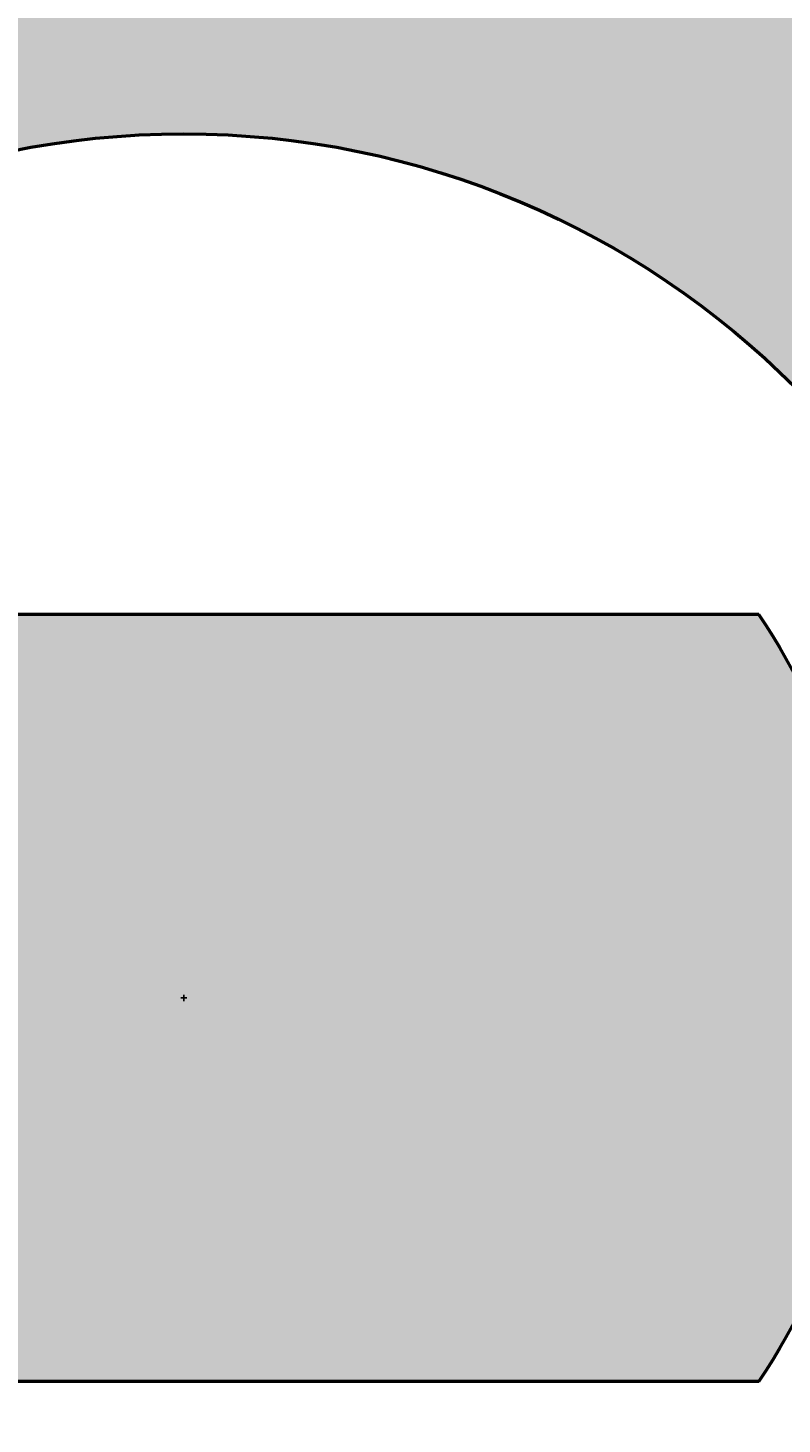
# Model space of a CAD drawing. Units: inches. Extents: x 139261 to 139415, y 52839 to 52963.
# Tile 14 of 20: x 139336 to 139358, y 52888 to 52928. Entities that reach past the tile are written whole.
import ezdxf

# ---------------------------------------------------------------- set-up
doc = ezdxf.new("R2010")
doc.units = ezdxf.units.IN
doc.header["$MEASUREMENT"] = 0
for name, color, linetype, lineweight in [('M-DIMS', 2, 'Continuous', 25), ('M-HATC', 8, 'Continuous', 18), ('M-OUTL', 7, 'Continuous', 50)]:
    doc.layers.add(name, color=color, linetype=linetype, lineweight=lineweight)
doc.styles.get("Standard").update_dxf_attribs({"font": 'arial.ttf'})
doc.dimstyles.get("Standard").update_dxf_attribs({"dimtxt": 0.18, "dimasz": 0.18, "dimexe": 0.18, "dimexo": 0.0625, "dimgap": 0.09, "dimtad": 0, "dimtih": 1, "dimtoh": 1, "dimdec": 4, "dimzin": 0, "dimdsep": 46, "dimtxsty": 'Standard', "dimcen": 0.09, "dimadec": 0, "dimazin": 0, "dimtfac": 1, "dimtdec": 4, "dimtofl": 0, "dimtmove": 0, "dimatfit": 3, "dimfxl": 1, "dimtolj": 1, "dimtzin": 0, "dimarcsym": 0})

# ---------------------------------------------------------------- blocks, each defined once
blk = doc.blocks.new('*D3')
at = {"layer": 'Defpoints', "color": 0, "transparency": 16777216}
for p in [(139359.484, 52906.062), (139321.23, 52894.373)]:
    blk.add_point(p, dxfattribs=at)
at = {"layer": 'M-DIMS', "color": 0, "lineweight": -2, "transparency": 16777216}
for p, q in [((139412.091, 52922.136), (139359.656, 52906.115)), ((139412.271, 52922.136), (139412.091, 52922.136)), ((139340.357, 52900.127), (139340.357, 52900.307)), ((139340.267, 52900.217), (139340.447, 52900.217))]:
    blk.add_line(p, q, dxfattribs=at)
at = {"layer": 'M-DIMS', "color": 0, "transparency": 16777216}
blk.add_solid([(139359.647, 52906.143), (139359.665, 52906.086), (139359.484, 52906.062)], dxfattribs=at)
at = {"layer": 'M-DIMS', "color": 0, "transparency": 16777216, "insert": (139412.902, 52922.136), "char_height": 0.18, "attachment_point": 5}
blk.add_mtext('\\A1;∅40.0000', dxfattribs=at)
blk = doc.blocks.new('*D4')
at = {"layer": 'Defpoints', "color": 0, "transparency": 16777216}
for p in [(139373.053, 52923.26), (139307.661, 52877.175)]:
    blk.add_point(p, dxfattribs=at)
at = {"layer": 'M-DIMS', "color": 0, "lineweight": -2, "transparency": 16777216}
for p, q in [((139414.011, 52952.126), (139373.2, 52923.364)), ((139414.191, 52952.126), (139414.011, 52952.126)), ((139340.357, 52900.127), (139340.357, 52900.307)), ((139340.267, 52900.217), (139340.447, 52900.217))]:
    blk.add_line(p, q, dxfattribs=at)
blk.add_arc((139340.357, 52900.217), 40, 34.9168, 52.0771, dxfattribs=at)
at = {"layer": 'M-DIMS', "color": 0, "transparency": 16777216}
blk.add_solid([(139373.183, 52923.388), (139373.217, 52923.339), (139373.053, 52923.26)], dxfattribs=at)
at = {"layer": 'M-DIMS', "color": 0, "transparency": 16777216, "insert": (139414.822, 52952.126), "char_height": 0.18, "attachment_point": 5}
blk.add_mtext('\\A1;∅80.0000', dxfattribs=at)
blk = doc.blocks.new('*D5')
at = {"layer": 'Defpoints', "color": 0, "transparency": 16777216}
for p in [(139316.763, 52908.484), (139363.951, 52891.951)]:
    blk.add_point(p, dxfattribs=at)
at = {"layer": 'M-DIMS', "color": 0, "lineweight": -2, "transparency": 16777216}
for p, q in [((139262.553, 52927.414), (139262.733, 52927.414)), ((139262.733, 52927.414), (139316.593, 52908.544)), ((139340.357, 52900.127), (139340.357, 52900.307)), ((139340.267, 52900.217), (139340.447, 52900.217))]:
    blk.add_line(p, q, dxfattribs=at)
at = {"layer": 'M-DIMS', "color": 0, "transparency": 16777216}
blk.add_solid([(139316.603, 52908.572), (139316.583, 52908.515), (139316.763, 52908.484)], dxfattribs=at)
at = {"layer": 'M-DIMS', "color": 0, "transparency": 16777216, "insert": (139261.922, 52927.414), "char_height": 0.18, "attachment_point": 5}
blk.add_mtext('\\A1;∅50.0000', dxfattribs=at)
blk = doc.blocks.new('*D6')
at = {"layer": 'Defpoints', "color": 0, "transparency": 16777216}
for p in [(139332.153, 52949.54), (139348.561, 52850.895)]:
    blk.add_point(p, dxfattribs=at)
at = {"layer": 'M-DIMS', "color": 0, "lineweight": -2, "transparency": 16777216}
for p, q in [((139329.787, 52962.682), (139329.967, 52962.682)), ((139329.967, 52962.682), (139332.124, 52949.717)), ((139340.357, 52900.127), (139340.357, 52900.307)), ((139340.267, 52900.217), (139340.447, 52900.217))]:
    blk.add_line(p, q, dxfattribs=at)
at = {"layer": 'M-DIMS', "color": 0, "transparency": 16777216}
blk.add_solid([(139332.153, 52949.722), (139332.094, 52949.713), (139332.153, 52949.54)], dxfattribs=at)
at = {"layer": 'M-DIMS', "color": 0, "transparency": 16777216, "insert": (139329.086, 52962.682), "char_height": 0.18, "attachment_point": 5}
blk.add_mtext('\\A1;∅100.0000', dxfattribs=at)
blk = doc.blocks.new('*D9')
at = {"layer": 'Defpoints', "color": 0, "transparency": 16777216}
for p in [(139302.054, 52932.357), (139378.659, 52868.078)]:
    blk.add_point(p, dxfattribs=at)
at = {"layer": 'M-DIMS', "color": 0, "lineweight": -2, "transparency": 16777216}
for p, q in [((139278.893, 52951.64), (139279.073, 52951.64)), ((139279.073, 52951.64), (139301.916, 52932.472)), ((139340.357, 52900.127), (139340.357, 52900.307)), ((139340.267, 52900.217), (139340.447, 52900.217))]:
    blk.add_line(p, q, dxfattribs=at)
at = {"layer": 'M-DIMS', "color": 0, "transparency": 16777216}
blk.add_solid([(139301.936, 52932.495), (139301.897, 52932.449), (139302.054, 52932.357)], dxfattribs=at)
at = {"layer": 'M-DIMS', "color": 0, "transparency": 16777216, "insert": (139278.506, 52951.64), "char_height": 0.18, "attachment_point": 5}
blk.add_mtext('\\A1;∅100', dxfattribs=at)
blk = doc.blocks.new('*D10')
at = {"layer": 'Defpoints', "color": 0, "transparency": 16777216}
for p in [(139325.07, 52937.181), (139355.644, 52863.254)]:
    blk.add_point(p, dxfattribs=at)
at = {"layer": 'M-DIMS', "color": 0, "lineweight": -2, "transparency": 16777216}
for p, q in [((139340.357, 52900.127), (139340.357, 52900.307)), ((139340.267, 52900.217), (139340.447, 52900.217)), ((139364.816, 52841.075), (139355.712, 52863.087)), ((139364.996, 52841.075), (139364.816, 52841.075))]:
    blk.add_line(p, q, dxfattribs=at)
at = {"layer": 'M-DIMS', "color": 0, "transparency": 16777216}
blk.add_solid([(139355.74, 52863.099), (139355.685, 52863.076), (139355.644, 52863.254)], dxfattribs=at)
at = {"layer": 'M-DIMS', "color": 0, "transparency": 16777216, "insert": (139365.312, 52841.075), "char_height": 0.18, "attachment_point": 5}
blk.add_mtext('\\A1;∅80', dxfattribs=at)

msp = doc.modelspace()

# ---------------------------------------------------------------- hatches: boundary and pattern name
at = {"layer": 'M-HATC'}
h = msp.add_hatch(color=256, dxfattribs=at)
h.dxf.hatch_style = 1
h.paths.add_polyline_path([(139290.35689, 52900.21749, 1), (139390.35689, 52900.21749, 1)])
h.paths.add_polyline_path([(139335.36666, 52939.90499, -0.01563646), (139335.35689, 52940.21749, -1), (139345.35689, 52940.21749, -0.01563646), (139345.34711, 52939.90499, -0.13461315), (139364.89157, 52931.80941, -0.691035), (139373.64116, 52928.50176, -0.21521822), (139371.94881, 52924.75216, -0.13461315), (139380.04439, 52905.20771, -0.43265224), (139385.35689, 52900.21749, -0.43265224), (139380.04439, 52895.22726, -0.13461315), (139371.94881, 52875.68281, -0.21521822), (139373.64116, 52871.93321, -0.691035), (139364.89157, 52868.62556, -0.13461315), (139345.34711, 52860.52999, -0.01563646), (139345.35689, 52860.21749, -1), (139335.35689, 52860.21749, -0.01563646), (139335.36666, 52860.52999, -0.13461315), (139315.82221, 52868.62556, -0.691035), (139307.07262, 52871.93321, -0.21521822), (139308.76496, 52875.68281, -0.13461315), (139300.66939, 52895.22726, -0.43265224), (139295.35689, 52900.21749, -0.43265224), (139300.66939, 52905.20771, -0.13461315), (139308.76496, 52924.75216, -0.21521822), (139307.07262, 52928.50176, -0.691035), (139315.82221, 52931.80941, -0.13461315)], flags=16)
h.paths.add_polyline_path([(139365.35689, 52900.21749, -1), (139315.35689, 52900.21749, -1)], flags=0)
h.paths.add_polyline_path([(139323.71474, 52911.30978), (139356.99903, 52911.30978, -0.3027197), (139356.99903, 52889.12519), (139323.71474, 52889.12519, -0.3027197)], flags=0)
h.paths.add_polyline_path([(139364.89157, 52931.80941, 0.13461315), (139345.34711, 52939.90499, -0.93933644), (139335.36666, 52939.90499, 0.13461315), (139315.82221, 52931.80941, -0.18270763), (139317.07262, 52928.50176, -0.64579494), (139308.76496, 52924.75216, 0.13461315), (139300.66939, 52905.20771, -0.39601219), (139305.35689, 52900.21749, -0.39601219), (139300.66939, 52895.22726, 0.13461315), (139308.76496, 52875.68281, -0.64579494), (139317.07262, 52871.93321, -0.18270763), (139315.82221, 52868.62556, 0.13461315), (139335.36666, 52860.52999, -0.93933644), (139345.34711, 52860.52999, 0.13461315), (139364.89157, 52868.62556, -0.18270763), (139363.64116, 52871.93321, -0.64579494), (139371.94881, 52875.68281, 0.13461315), (139380.04439, 52895.22726, -0.39601219), (139375.35689, 52900.21749, -0.39601219), (139380.04439, 52905.20771, 0.13461315), (139371.94881, 52924.75216, -0.64579494), (139363.64116, 52928.50176, -0.18270763)], flags=0)
h = msp.add_hatch(color=256, dxfattribs=at)
h.dxf.hatch_style = 1
h.paths.add_polyline_path([(139345.34711, 52939.90499, -0.93933644), (139335.36666, 52939.90499, 0.13461315), (139315.82221, 52931.80941, -0.18270763), (139317.07262, 52928.50176, -0.64579494), (139308.76496, 52924.75216, 0.13461315), (139300.66939, 52905.20771, -0.39601219), (139305.35689, 52900.21749, -0.39601219), (139300.66939, 52895.22726, 0.13461315), (139308.76496, 52875.68281, -0.64579494), (139317.07262, 52871.93321, -0.18270763), (139315.82221, 52868.62556, 0.13461315), (139335.36666, 52860.52999, -0.93933644), (139345.34711, 52860.52999, 0.13461315), (139364.89157, 52868.62556, -0.18270763), (139363.64116, 52871.93321, -0.64579494), (139371.94881, 52875.68281, 0.13461315), (139380.04439, 52895.22726, -0.39601219), (139375.35689, 52900.21749, -0.39601219), (139380.04439, 52905.20771, 0.13461315), (139371.94881, 52924.75216, -0.64579494), (139363.64116, 52928.50176, -0.18270763), (139364.89157, 52931.80941, 0.13461315)])
h.paths.add_polyline_path([(139365.35689, 52900.21749, -1), (139315.35689, 52900.21749, -1)], flags=16)
h.paths.add_polyline_path([(139356.99903, 52911.30978, -0.3027197), (139356.99903, 52889.12519), (139323.71474, 52889.12519, -0.3027197), (139323.71474, 52911.30978)], flags=0)
h = msp.add_hatch(color=256, dxfattribs=at)
h.dxf.hatch_style = 1
h.paths.add_polyline_path([(139356.99903, 52911.30978), (139323.71474, 52911.30978, 0.3027197), (139323.71474, 52889.12519), (139356.99903, 52889.12519, 0.3027197)])

# ---------------------------------------------------------------- linework, layer by layer
at = {"layer": 'M-OUTL'}
for p, q in [((139356.99903, 52911.30978), (139323.71474, 52911.30978)), ((139356.99903, 52889.12519), (139323.71474, 52889.12519))]:
    msp.add_line(p, q, dxfattribs=at)
for radius in [50, 25]:
    msp.add_circle((139340.35689, 52900.21749), radius, dxfattribs=at)
msp.add_arc((139340.35689, 52900.21749), 20, 326.315805, 33.684195, dxfattribs=at)

# ---------------------------------------------------------------- dimensions: what is measured, and where the dimension line sits
at = {"layer": 'M-DIMS'}
for p1, p2, override, picture, middle in [((139348.56051, 52850.89507), (139332.15326, 52949.5399), {"dimclrd": 0, "dimclre": 0, "dimclrt": 0}, '*D6', (139329.08622, 52962.68242)), ((139307.66087, 52877.17469), (139373.0529, 52923.26028), {"dimclrd": 0, "dimclre": 0, "dimclrt": 0}, '*D4', (139414.82217, 52952.12585)), ((139378.65939, 52868.07845), (139302.05438, 52932.35652), {"dimdec": 0, "dimlfac": 1, "dimrnd": 0, "dimzin": 0, "dimdsep": 46, "dimlunit": 2}, '*D9', (139278.50641, 52951.63995)), ((139325.07023, 52937.18123), (139355.64354, 52863.25374), {"dimdec": 0, "dimlfac": 1, "dimrnd": 0, "dimzin": 0, "dimdsep": 46, "dimlunit": 2}, '*D10', (139365.31206, 52841.0755)), ((139363.95063, 52891.95098), (139316.76314, 52908.48399), {"dimclrd": 0, "dimclre": 0, "dimclrt": 0}, '*D5', (139261.92224, 52927.41429)), ((139321.22987, 52894.37307), (139359.4839, 52906.0619), {"dimclrd": 0, "dimclre": 0, "dimclrt": 0}, '*D3', (139412.90184, 52922.13633))]:
    dim = msp.add_diameter_dim_2p(p1=p1, p2=p2, dimstyle='Standard', override=override, dxfattribs=at)
    dim.commit()
    dim.dimension.update_dxf_attribs({"geometry": picture, "text_midpoint": middle, "dimtype": 163})

doc.saveas('drawing.dxf')
